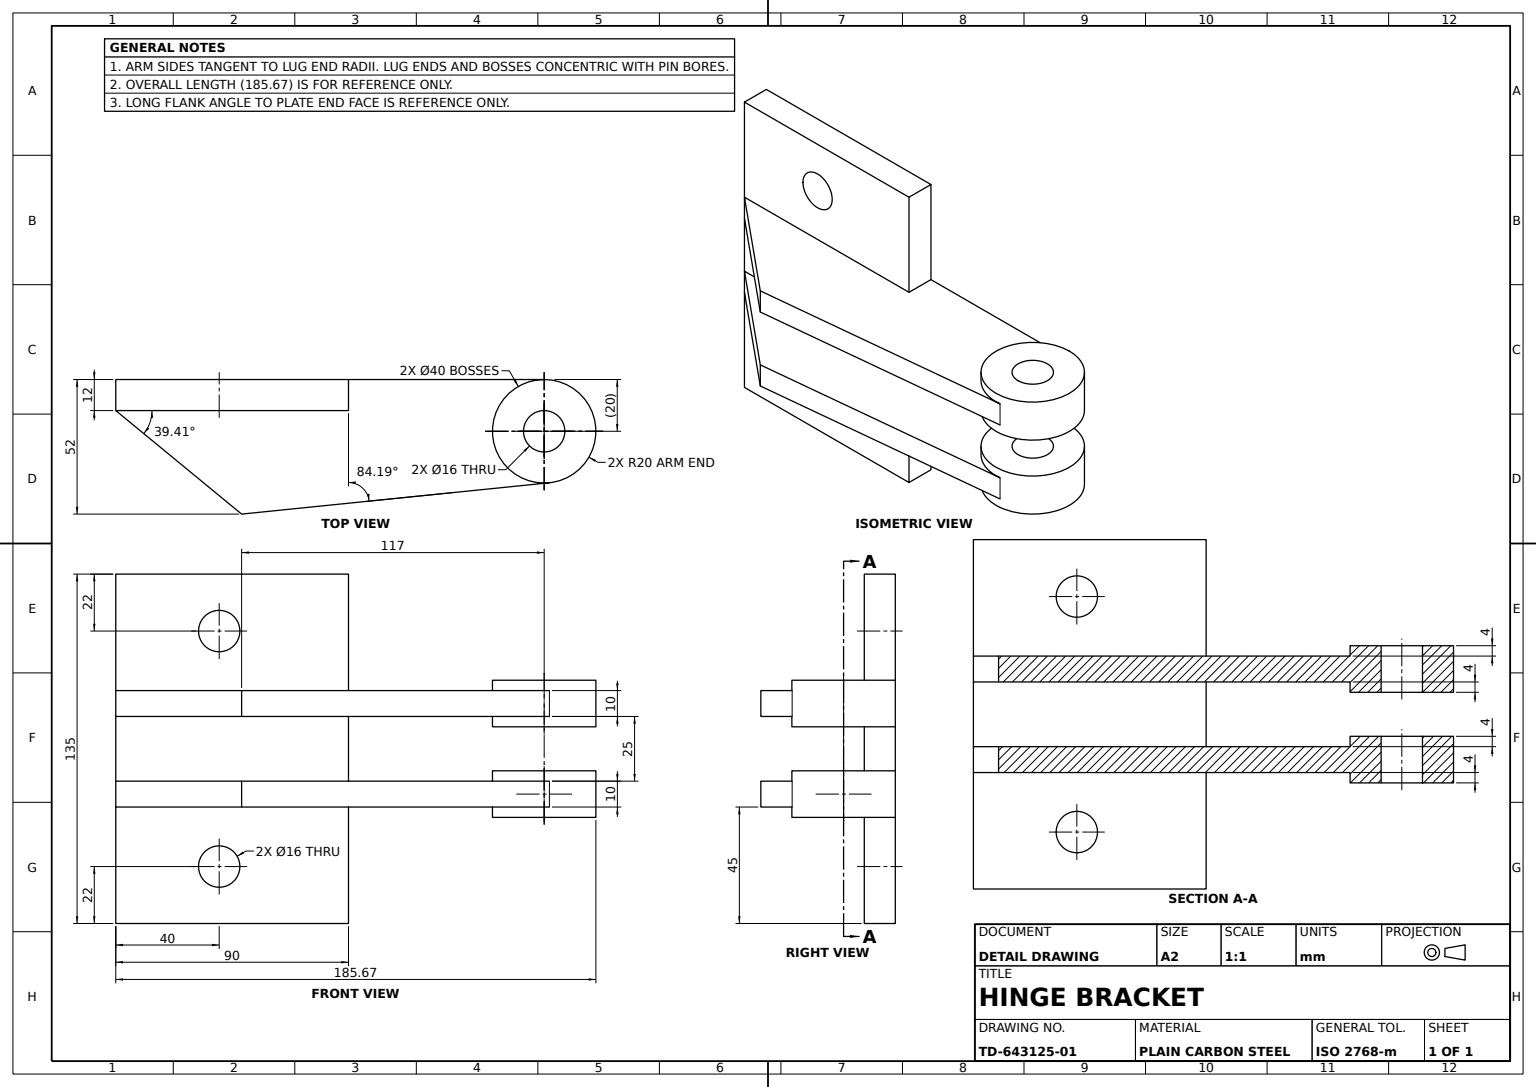
SolidWorks part; units mm, degrees
material "Plain Carbon Steel"
ref_plane "Front Plane" through (0, 0, 0) normal (0, 0, 1) x (1, 0, 0)
ref_plane "Top Plane" through (0, 0, 0) normal (0, 1, 0) x (1, 0, 0)
ref_plane "Right Plane" through (0, 0, 0) normal (1, 0, 0) x (0, 0, -1)
sketch "Base Plate Sketch" plane through (0, 0, 0) normal (0, 0, 1) x (1, 0, 0)
  line L0 (-203.6725, 0) -> (172.1836, 0) construction
  line L1 (0, 116.0732) -> (0, -122.773) construction
  line L3 (-45, -67.5) -> (45, -67.5)
  line L4 (-45, -67.5) -> (-45, 67.5)
  line L5 (-45, 67.5) -> (45, 67.5)
  line L6 (45, -67.5) -> (45, 67.5)
  line L7 (-45, -67.5) -> (45, 67.5) construction
  line L8 (-45, 67.5) -> (45, -67.5) construction
  point P5 (0, 0)
  dimension "D1" = 135
  dimension "D2" = 90
extrude "Base Plate" add sketch "Base Plate Sketch" along normal blind 12
sketch "Mounting Holes Sketch" plane through (0, 0, 12) normal (0, 0, 1) x (1, 0, 0)
  line L0 (45, -67.5) -> (45, 67.5) construction
  line L1 (-45, -67.5) -> (45, -67.5) construction
  line L2 (45, 67.5) -> (-45, 67.5) construction
  circle A0 centre (5, -45.5) radius 8
  circle A1 centre (5, 45.5) radius 8
  dimension "D1" = 40
  dimension "D2" = 22
  dimension "D3" = 16
  dimension "D4" = 40
  dimension "D5" = 22
  dimension "D6" = 16
extrude "Mounting Holes 2xØ16" cut sketch "Mounting Holes Sketch" against normal blind 22
sketch "Clevis Arm Sketch" plane through (0, 0, 0) normal (0, 1, 0) x (1, 0, 0)
  line L1 (-45, -12) -> (-120.6724, -12)
  line L2 (45, 0) -> (-3.6724, 40)
  line L3 (45, -12) -> (-45, -12) construction
  line L4 (-3.6724, 40) -> (-122.6956, 27.8974)
  line L5 (-45, -12) -> (-45, 0) construction
  line L6 (-45, -12) -> (-45, 0)
  line L7 (45, 0) -> (-45, 0) construction
  line L8 (45, 0) -> (-45, 0)
  circle A0 centre (-120.6724, 8) radius 8
  circle A1 centre (-120.6724, 8) radius 20
  dimension "D1" = 40
  dimension "D2" = 16
  dimension "D3" = 52
  dimension "D4" = 63
  dimension "D5" = 117
extrude "Clevis Arm" add sketch "Clevis Arm Sketch" along normal mid plane 45 contours A1 L1 L6 L8 L2 L4 | A1 A0
sketch "Clevis Slot Sketch" plane through (0, 0, 0) normal (1, 0, 0) x (0, 0, -1)
  line L0 (-30.1327, 0) -> (75.4841, 0) construction
  line L1 (0, -12.5) -> (40, -12.5)
  line L2 (0, 12.5) -> (40, 12.5)
  line L3 (40, 22.5) -> (40, -22.5) construction
  line L4 (40, 12.5) -> (40, -12.5)
  line L5 (0, 22.5) -> (0, -22.5) construction
  line L6 (0, 12.5) -> (0, -12.5)
  line L8 (-30.1327, 12.5) -> (75.4841, 12.5) construction
  line L9 (-30.1327, -12.5) -> (75.4841, -12.5) construction
  dimension "D1" = 12.5
  dimension "D2" = 12.5
extrude "Clevis Slot" cut sketch "Clevis Slot Sketch" against normal through all both and the other way through all
sketch "Pin Hole Sketch" plane through (0, 0, 12) normal (0, 0, 1) x (1, 0, 0)
  line L0 (-179.3249, 0) -> (54.7892, 0) construction
  line L1 (-45, 12.5) -> (-45, -12.5)
  line L2 (-139.0027, 12.5) -> (-45, 12.5)
  line L3 (-139.0027, -12.5) -> (-45, -12.5)
  line L4 (-139.0027, 12.5) -> (-139.0027, -12.5) construction
  line L5 (-139.0027, 12.5) -> (-139.0027, -12.5)
  dimension "D1" = 45
extrude "Pin Hole" cut sketch "Pin Hole Sketch" against normal through all both
sketch "Lug Boss 1 Sketch" plane through (0, -22.5, 0) normal (0, -1, 0) x (1, 0, 0)
  circle A0 centre (-120.6724, -8) radius 20
  circle A1 centre (-120.6724, -8) radius 8
  dimension "D1" = 40
  dimension "D2" = 16
extrude "Lug Boss 1 Ø40" add sketch "Lug Boss 1 Sketch" along normal blind 4
sketch "Lug Boss 2 Sketch" plane through (0, -12.5, 0) normal (0, 1, 0) x (1, 0, 0)
  circle A0 centre (-120.6724, 8) radius 20
  circle A1 centre (-120.6724, 8) radius 8
  dimension "D1" = 40
  dimension "D2" = 16
extrude "Lug Boss 2 Ø40" add sketch "Lug Boss 2 Sketch" along normal blind 4
sketch "Lug Boss 3 Sketch" plane through (0, 22.5, 0) normal (0, 1, 0) x (1, 0, 0)
  circle A0 centre (-120.6724, 8) radius 20
  circle A1 centre (-120.6724, 8) radius 8
  dimension "D1" = 40
  dimension "D2" = 16
extrude "Lug Boss 3 Ø40" add sketch "Lug Boss 3 Sketch" along normal blind 4
sketch "Lug Boss 4 Sketch" plane through (0, 12.5, 0) normal (0, -1, 0) x (1, 0, 0)
  circle A0 centre (-120.6724, -8) radius 8
  circle A1 centre (-120.6724, -8) radius 20
  dimension "D1" = 40
  dimension "D2" = 16
extrude "Lug Boss 4 Ø40" add sketch "Lug Boss 4 Sketch" along normal blind 4
